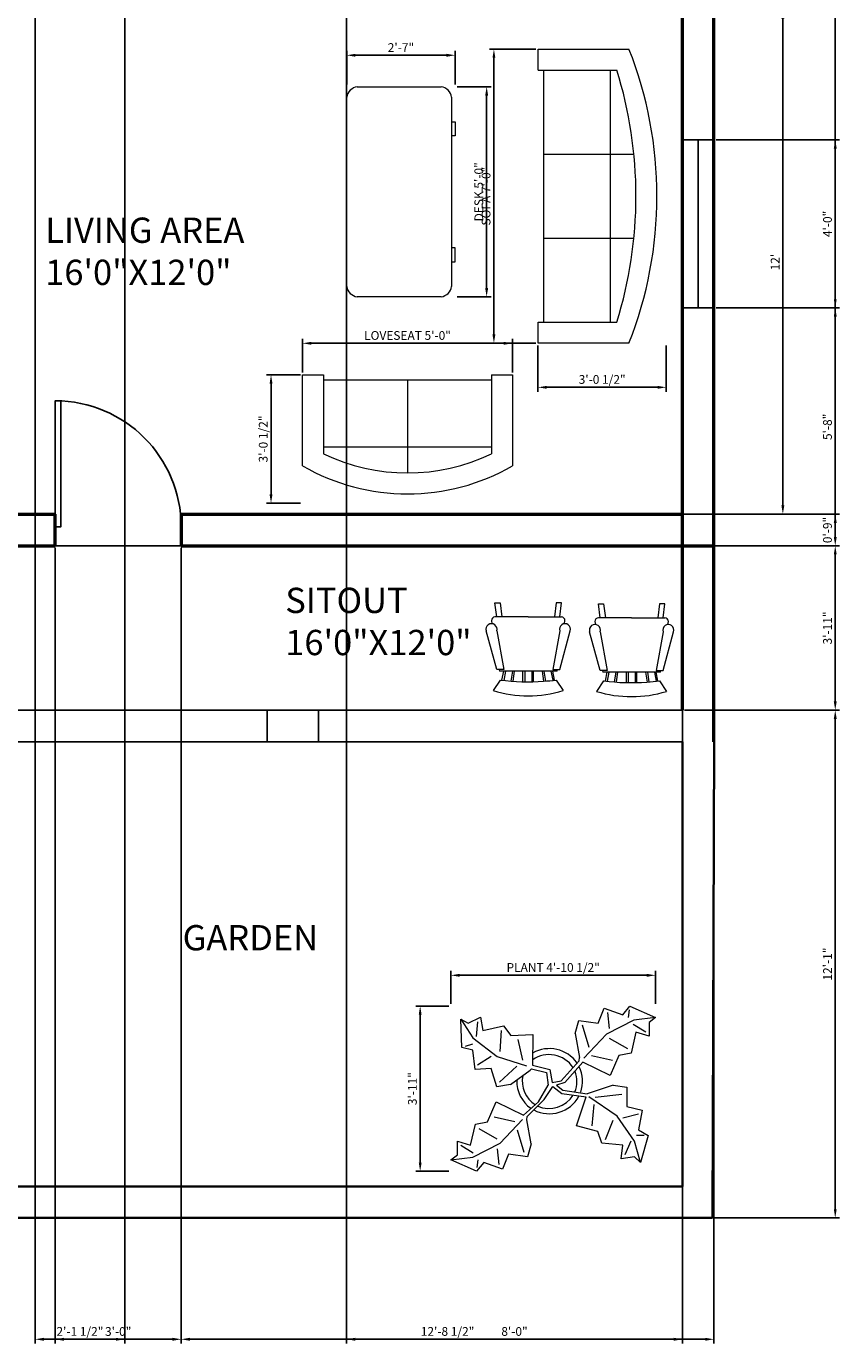
# Model space of a CAD drawing. Units: inches. Extents: x 25547 to 25983, y 30413 to 31159.
# Tile 2 of 5: x 25750 to 25982, y 30413 to 30790. Entities that reach past the tile are written whole.
import ezdxf

# ---------------------------------------------------------------- set-up
doc = ezdxf.new("R2010")
doc.units = ezdxf.units.IN
for name, color, linetype, lineweight in [('A-AREA-IDEN', 11, 'Continuous', 25), ('A-FLOR-PORC', 151, 'Continuous', 25), ('A-WALL', 7, 'Continuous', 50), ('DIM', 4, 'Continuous', 18), ('DOOR', 3, 'Continuous', 25), ('FLOWER', 60, 'Continuous', 13), ('FURNITURES', 6, 'Continuous', 18), ('L-SITE-WALL', 7, 'Continuous', 35), ('WINDOW', 1, 'Continuous', 25)]:
    doc.layers.add(name, color=color, linetype=linetype, lineweight=lineweight)
doc.styles.get("Standard").update_dxf_attribs({"font": 'arial.ttf'})
doc.dimstyles.new('ISO-25', dxfattribs={"dimtxt": 2.5, "dimasz": 2.5, "dimexe": 1.25, "dimexo": 0.625, "dimtad": 1, "dimlunit": 3, "dimtxsty": 'Standard', "dimcen": 2.5, "dimadec": 0, "dimazin": 0, "dimtfac": 1, "dimtmove": 0, "dimatfit": 3, "dimfxl": 1, "dimarcsym": 0})

# ---------------------------------------------------------------- blocks, each defined once
blk = doc.blocks.new('*U2')
for p, q in [((0, 0), (0, -6)), ((40, 0), (40, -6))]:
    blk.add_line(p, q)
blk.add_lwpolyline([(0, 0), (0, 40), (1.75, 40), (1.75, 0)], close=True)
blk.add_arc((0, 0), 40, 0, 90)
blk = doc.blocks.new('Desk - 30 x 60 in.')
for p, q in [((-26.999995, 0), (26.999995, 0)), ((-29.999995, -27), (-29.999995, -3)), ((29.999995, -3), (29.999995, -27)), ((26.999995, -30), (-26.999995, -30)), ((-20.000005, -30), (-20.000005, -31)), ((-16.000005, -31), (-16.000005, -30)), ((15.999995, -31), (15.999995, -30)), ((19.999995, -30), (19.999995, -31)), ((-20.000005, -31), (-16.000005, -31)), ((19.999995, -31), (15.999995, -31))]:
    blk.add_line(p, q)
for centre, start, end in [((-26.499995, -3.5), 98.1301, 171.8699), ((26.499995, -3.5), 8.130102, 81.8699), ((-26.499995, -26.5), 188.1301, 261.8699), ((26.499995, -26.5), 278.1301, 351.8699)]:
    blk.add_arc(centre, 3.535534, start, end)
blk = doc.blocks.new('Sofa - Roundback 7 ft.')
for p, q in [((-12.00002, -32.4421), (-12.00003, -6.5971)), ((11.99997, -32.4421), (11.99998, -6.5971)), ((-36.000027, -34), (-36.000027, -11.4696)), ((-35.999844, -13.3819), (35.9998, -13.3819)), ((35.99998, -34), (35.99998, -11.4696)), ((-36.000027, -32.4421), (35.99998, -32.4421))]:
    blk.add_line(p, q)
for points in [[(-36.000027, -34), (-42.000027, -34), (-42.000027, -8)], [(41.99998, -8), (41.99998, -34), (35.99998, -34)]]:
    blk.add_lwpolyline(points)
for centre, radius, start, end in [((0, -114.25), 114.25, 68.43141, 111.5686), ((-0.00001, -127.1968), 121.1968, 72.72033, 107.2797)]:
    blk.add_arc(centre, radius, start, end)
blk = doc.blocks.new('Sofa - Roundback Loveseat 5 ft.')
for p, q in [((0, -32.44198), (0, -5.99998)), ((-24, -33.99998), (-24, -11.46958)), ((-23.9998, -13.38178), (23.99986, -13.38178)), ((24.00004, -33.99998), (24.00004, -11.46958)), ((-24, -32.44198), (24.00004, -32.44198))]:
    blk.add_line(p, q)
for points in [[(-24, -33.99998), (-30, -33.99998), (-30, -7.99998)], [(30.00004, -7.99998), (30.00004, -33.99998), (24.00004, -33.99998)]]:
    blk.add_lwpolyline(points)
for centre, radius, start, end in [((0, -60.24998), 60.24998, 60.13715, 119.8628), ((0, -61.38438), 55.38444, 64.32083, 115.6792)]:
    blk.add_arc(centre, radius, start, end)
blk = doc.blocks.new('Plant - Rubber or Philodendron')
for p, q in [((8.8871, 10.7908), (9.9809, 13.4933)), ((9.9809, 13.4933), (13.3837, 12.301)), ((10.5828, 12.6946), (10.8893, 9.7953)), ((13.3837, 12.301), (14.68, 13.9039)), ((14.5816, 13.2037), (14.3848, 11.8033)), ((14.68, 13.9039), (19.3848, 11.8146)), ((-16.2005, 11.4774), (-13.9899, 8.1064)), ((-16.2005, 11.4774), (-14.8639, 10.7964)), ((-16.0159, 6.3329), (-16.2005, 11.4774)), ((-14.8639, 10.7964), (-12.6195, 11.8975)), ((-13.3174, 8.325), (-13.0735, 11.0065)), ((-12.6195, 11.8975), (-12.1909, 9.4345)), ((-12.1909, 9.4345), (-8.3829, 10.3)), ((-8.3829, 10.3), (-7.0549, 8.501)), ((4.6914, 8.8812), (5.3859, 11.2828)), ((5.3859, 11.2828), (8.8871, 10.7908)), ((5.9878, 10.4842), (7.1971, 6.3869)), ((15.3859, 11.3055), (10.3916, 8.7942)), ((15.2875, 10.6053), (17.5907, 9.2105)), ((19.3848, 11.8146), (15.3859, 11.3055)), ((19.3848, 11.8146), (18.1868, 10.9119)), ((18.1868, 10.9119), (18.1925, 8.4119)), ((-13.9899, 8.1064), (-9.5434, 4.7185)), ((-8.8369, 9.409), (-9.0894, 5.6095)), ((-7.0549, 8.501), (-3.0284, 8.6941)), ((-4.8529, 4.012), (-5.7184, 7.82)), ((-3.0284, 8.6941), (-3.0709, 3.1041)), ((4.6914, 8.8812), (5.5014, 4.4831)), ((10.3916, 8.7942), (6.2847, 4.4028)), ((14.2977, 6.1031), (10.9934, 7.9956)), ((15.7909, 9.1065), (14.8995, 5.3044)), ((18.1925, 8.4119), (15.7909, 9.1065)), ((-14.0069, 5.8704), (-16.0159, 6.3329)), ((-15.3434, 6.5514), (-13.9984, 6.9884)), ((-13.5868, 2.2894), (-14.0069, 5.8704)), ((7.7005, 4.8881), (11.5025, 3.9967)), ((12.7005, 4.8994), (11.1089, 1.1958)), ((14.8995, 5.3044), (12.7005, 4.8994)), ((-10.6784, 2.491), (-13.5868, 2.2894)), ((-13.1329, 3.1804), (-10.6614, 4.727)), ((-9.5858, -0.8715), (-10.6784, 2.491)), ((-9.5434, 4.7185), (-4.1917, 2.9888)), ((-9.1318, 0.0195), (-5.9793, 2.9025)), ((-3.5248, 2.2131), (-3.3011, 2.4355)), ((-3.3011, 2.4355), (-0.5306, 1.7947)), ((-3.0709, 3.1041), (0.0797, 2.3163)), ((2.1141, 0.2298), (5.4346, 3.9146)), ((6.1032, 3.6844), (2.8262, -0.031)), ((5.4346, 3.9146), (5.5014, 4.4831)), ((11.1089, 1.1958), (6.1032, 3.6844)), ((-7.1228, -0.443), (-3.5248, 2.2131)), ((-0.5306, 1.7947), (-0.2255, -0.5527)), ((-0.5306, 1.7947), (-0.5306, 1.7947)), ((0.0797, 2.3163), (0.4866, -0.031)), ((0.4866, -0.031), (2.1141, 0.2298)), ((-7.1228, -0.443), (-9.5858, -0.8715)), ((-2.019, -3.6148), (-0.2255, -0.5527)), ((-0.9375, -3.1608), (0.5883, -0.8135)), ((0.5883, -0.8135), (2.2447, -2.0916)), ((2.8262, -0.031), (1.3003, -0.5527)), ((1.3003, -0.5527), (2.4193, -1.4655)), ((2.2447, -2.0916), (6.7108, -2.6626)), ((2.4193, -1.4655), (6.895, -2.1175)), ((11.6605, -0.5413), (6.895, -2.1175)), ((8.3544, -2.7453), (13.1973, -2.1704)), ((11.6605, -0.5413), (14.1354, -0.8948)), ((14.1354, -0.8948), (14.1354, -4.4304)), ((-11.3237, -7.2629), (-9.7321, -3.5593)), ((-9.7321, -3.5593), (-4.7264, -6.0479)), ((-2.019, -3.6148), (-4.7264, -6.0479)), ((-4.0579, -6.2781), (-0.9375, -3.1608)), ((4.943, -7.9659), (6.7108, -2.6626)), ((12.3677, -6.1981), (7.219, -2.6772)), ((8.125, -4.0768), (7.7715, -7.9659)), ((14.1354, -4.4304), (16.9638, -5.1375)), ((-6.3237, -7.2516), (-10.1257, -6.3602)), ((-9.0148, -11.1577), (-4.9047, -6.8122)), ((-4.1246, -6.8466), (-4.0579, -6.2781)), ((-3.3146, -11.2447), (-4.1246, -6.8466)), ((10.2463, -10.4408), (11.6605, -6.9053)), ((15.5496, -10.7943), (12.3677, -6.1981)), ((16.2567, -5.8446), (13.4283, -6.5517)), ((16.9638, -5.1375), (16.2567, -8.673)), ((-14.4141, -11.4699), (-13.5228, -7.6679)), ((-13.5228, -7.6679), (-11.3237, -7.2629)), ((-12.921, -8.4665), (-9.6166, -10.359)), ((-4.611, -12.8477), (-5.8203, -8.7504)), ((8.8321, -9.0266), (4.943, -7.9659)), ((9.5392, -11.1479), (8.8321, -9.0266)), ((16.2567, -8.673), (18.0245, -9.7337)), ((-16.8157, -10.7754), (-14.4141, -11.4699)), ((-16.8101, -13.2754), (-16.8157, -10.7754)), ((-13.9107, -12.9688), (-16.2139, -11.574)), ((-14.0091, -13.669), (-9.0148, -11.1577)), ((-3.3146, -11.2447), (-4.0092, -13.6463)), ((13.4283, -11.5015), (9.5392, -11.1479)), ((13.0748, -13.9763), (13.4283, -11.5015)), ((14.8425, -10.7943), (13.7819, -13.2692)), ((16.6103, -14.6834), (15.5496, -10.7943)), ((17.3174, -9.7337), (15.9032, -9.7337)), ((18.0245, -9.7337), (16.6103, -14.6834)), ((-18.008, -14.1781), (-16.8101, -13.2754)), ((-18.008, -14.1781), (-14.0091, -13.669)), ((-13.3032, -16.2674), (-18.008, -14.1781)), ((-13.2048, -15.5672), (-13.008, -14.1668)), ((-9.206, -15.0581), (-9.5126, -12.1588)), ((-7.5103, -13.1543), (-8.6042, -15.8568)), ((-4.0092, -13.6463), (-7.5103, -13.1543)), ((15.5496, -13.6228), (13.0748, -13.9763)), ((16.6103, -14.6834), (15.5496, -13.6228)), ((-12.0069, -14.6645), (-13.3032, -16.2674)), ((-8.6042, -15.8568), (-12.0069, -14.6645))]:
    blk.add_line(p, q)
for centre, radius, start, end in [((0, 0), 6.1275, 34.37569, 120.1028), ((-0.0601, -0.2075), 5.2461, 33.82192, 124.9414), ((-0.098, 0.1364), 6.1288, 341.2017, 26.09184), ((0.0308, 0.1664), 6, 178.6147, 235.1169), ((0.0308, 0.1664), 5, 168.1647, 238.6725), ((-0.2664, 0.1682), 5.2775, 338.4094, 20.03007), ((-0.1102, 0.4886), 5.2883, 247.3711, 327.472), ((-0.0234, 0.3825), 6.1492, 242.5812, 331.2714)]:
    blk.add_arc(centre, radius, start, end)
blk = doc.blocks.new('Chair - Rocking')
for p, q in [((-8, -4.5), (-10, -1.5)), ((8, -4.5), (10, -1.5)), ((-9, -7.5), (-12, -18.49999)), ((-7, -7.5), (-9, -7.5)), ((-9, -18.49999), (-7, -7.5)), ((-8.23428, -6.99939), (-8.3093, -7.47958)), ((-8.23041, -7), (8.23915, -7)), ((-7.5, -4.5), (-7, -7)), ((-6.5, -7), (-7.02225, -4.43)), ((-4.5, -7), (-4.96674, -4.19951)), ((-4, -7), (-4.40532, -4.16272)), ((-1.5, -4.05012), (-1.5, -7)), ((-1, -7), (-1, -4.05012)), ((1, -7), (1, -4.04655)), ((1.5, -4.05012), (1.5, -7)), ((4, -7), (4.40187, -4.18694)), ((4.5, -7), (4.96761, -4.19437)), ((6.5, -7), (7, -4.4057)), ((7.5, -4.5), (7, -7)), ((7, -7.5), (9, -7.5)), ((9, -18.49999), (7, -7.5)), ((8.31071, -7.48854), (8.23449, -7.00073)), ((9, -7.5), (12, -18.49999)), ((-10.36644, -20.64523), (-10.5, -21.49999)), ((-9, -22.49999), (-9.5, -26.49999)), ((0, -22.49999), (-9.5, -22.49999)), ((-8, -26.49999), (-7.5, -22.49999)), ((0, -22.49999), (9.5, -22.49999)), ((8, -26.49999), (7.5, -22.49999)), ((9, -22.49999), (9.5, -26.49999)), ((10.5, -21.49999), (10.3575, -20.58798)), ((-9.5, -26.49999), (-8, -26.49999)), ((9.5, -26.49999), (8, -26.49999))]:
    blk.add_line(p, q)
for centre, radius, start, end in [((0, -34.08333), 34.08333, 72.93847, 107.0615), ((0, -68.25004), 64.25, 93.92211, 97.15267), ((0, -68.25004), 64.25, 82.84733, 93.92211), ((-10.5, -18.99999), 1.58114, 161.5651, 18.43495), ((10.5, -18.99999), 1.58114, 161.5651, 18.43495), ((-9.5, -21.49999), 1, 180, 270), ((9.5, -21.49999), 1, 270, 0)]:
    blk.add_arc(centre, radius, start, end)
blk = doc.blocks.new('*D28')
at = {"layer": 'Defpoints', "color": 0, "transparency": 16777216}
for p in [(25937.53, 30794.83), (25966.22, 30794.83), (25937.53, 30650.83)]:
    blk.add_point(p, dxfattribs=at)
at = {"layer": 'DIM', "color": 0, "lineweight": -2, "transparency": 16777216}
for p, q in [((25938.15, 30794.83), (25967.47, 30794.83)), ((25966.22, 30653.33), (25966.22, 30792.33)), ((25938.15, 30650.83), (25967.47, 30650.83))]:
    blk.add_line(p, q, dxfattribs=at)
at = {"layer": 'DIM', "color": 0, "transparency": 16777216}
for points in [[(25965.8, 30792.33), (25966.63, 30792.33), (25966.22, 30794.83)], [(25965.8, 30653.33), (25966.63, 30653.33), (25966.22, 30650.83)]]:
    blk.add_solid(points, dxfattribs=at)
at = {"layer": 'DIM', "color": 0, "transparency": 16777216, "insert": (25964.34, 30722.83), "char_height": 2.5, "attachment_point": 5, "rotation": 90}
blk.add_mtext("12'", dxfattribs=at)
blk = doc.blocks.new('WIN-48IN')
blk.add_line((4.5, 48), (4.5, 0))
blk.add_lwpolyline([(0, 48), (9, 48), (9, 0), (0, 0)], close=True)
blk = doc.blocks.new('*D48')
at = {"layer": 'Defpoints', "color": 0, "transparency": 16777216}
for p in [(25929.84, 30519.14), (25871.35, 30510.37), (25929.84, 30510.37)]:
    blk.add_point(p, dxfattribs=at)
at = {"layer": 'DIM', "color": 0, "lineweight": -2, "transparency": 16777216}
for p, q in [((25871.35, 30510.99), (25871.35, 30520.39)), ((25929.84, 30510.99), (25929.84, 30520.39)), ((25873.85, 30519.14), (25927.34, 30519.14))]:
    blk.add_line(p, q, dxfattribs=at)
at = {"layer": 'DIM', "color": 0, "transparency": 16777216}
for points in [[(25873.85, 30519.56), (25873.85, 30518.72), (25871.35, 30519.14)], [(25927.34, 30519.56), (25927.34, 30518.72), (25929.84, 30519.14)]]:
    blk.add_solid(points, dxfattribs=at)
at = {"layer": 'DIM', "color": 0, "transparency": 16777216, "insert": (25900.59, 30521.06), "char_height": 2.5, "attachment_point": 5}
blk.add_mtext('PLANT 4\'-10 1/2"', dxfattribs=at)
blk = doc.blocks.new('*D49')
at = {"layer": 'Defpoints', "color": 0, "transparency": 16777216}
for p in [(25862.57, 30510.37), (25871.35, 30510.37), (25871.35, 30463.17)]:
    blk.add_point(p, dxfattribs=at)
at = {"layer": 'DIM', "color": 0, "lineweight": -2, "transparency": 16777216}
for p, q in [((25870.72, 30510.37), (25861.32, 30510.37)), ((25862.57, 30465.67), (25862.57, 30507.87)), ((25870.72, 30463.17), (25861.32, 30463.17))]:
    blk.add_line(p, q, dxfattribs=at)
at = {"layer": 'DIM', "color": 0, "transparency": 16777216}
for points in [[(25862.16, 30507.87), (25862.99, 30507.87), (25862.57, 30510.37)], [(25862.16, 30465.67), (25862.99, 30465.67), (25862.57, 30463.17)]]:
    blk.add_solid(points, dxfattribs=at)
at = {"layer": 'DIM', "color": 0, "transparency": 16777216, "insert": (25860.67, 30486.77), "char_height": 2.5, "attachment_point": 5, "rotation": 90}
blk.add_mtext('3\'-11"', dxfattribs=at)
blk = doc.blocks.new('*D58')
at = {"layer": 'Defpoints', "color": 0, "transparency": 16777216}
for p in [(25872.57, 30772.91), (25881.57, 30772.91), (25872.57, 30712.91)]:
    blk.add_point(p, dxfattribs=at)
at = {"layer": 'DIM', "color": 0, "lineweight": -2, "transparency": 16777216}
for p, q in [((25873.19, 30772.91), (25882.82, 30772.91)), ((25881.57, 30715.41), (25881.57, 30770.41)), ((25873.19, 30712.91), (25882.82, 30712.91))]:
    blk.add_line(p, q, dxfattribs=at)
at = {"layer": 'DIM', "color": 0, "transparency": 16777216}
for points in [[(25881.15, 30770.41), (25881.99, 30770.41), (25881.57, 30772.91)], [(25881.15, 30715.41), (25881.99, 30715.41), (25881.57, 30712.91)]]:
    blk.add_solid(points, dxfattribs=at)
at = {"layer": 'DIM', "color": 0, "transparency": 16777216, "insert": (25879.65, 30742.91), "char_height": 2.5, "attachment_point": 5, "rotation": 90}
blk.add_mtext('DESK 5\'-0"', dxfattribs=at)
blk = doc.blocks.new('*D59')
at = {"layer": 'Defpoints', "color": 0, "transparency": 16777216}
for p in [(25841.57, 30781.91), (25841.57, 30772.91), (25872.57, 30772.91)]:
    blk.add_point(p, dxfattribs=at)
at = {"layer": 'DIM', "color": 0, "lineweight": -2, "transparency": 16777216}
for p, q in [((25841.57, 30773.53), (25841.57, 30783.16)), ((25872.57, 30773.53), (25872.57, 30783.16)), ((25870.07, 30781.91), (25844.07, 30781.91))]:
    blk.add_line(p, q, dxfattribs=at)
at = {"layer": 'DIM', "color": 0, "transparency": 16777216}
for points in [[(25844.07, 30782.33), (25844.07, 30781.49), (25841.57, 30781.91)], [(25870.07, 30782.33), (25870.07, 30781.49), (25872.57, 30781.91)]]:
    blk.add_solid(points, dxfattribs=at)
at = {"layer": 'DIM', "color": 0, "transparency": 16777216, "insert": (25857.07, 30783.79), "char_height": 2.5, "attachment_point": 5}
blk.add_mtext('2\'-7"', dxfattribs=at)
blk = doc.blocks.new('*D62')
at = {"layer": 'Defpoints', "color": 0, "transparency": 16777216}
for p in [(25896.24, 30783.68), (25883.64, 30699.68), (25896.24, 30699.68)]:
    blk.add_point(p, dxfattribs=at)
at = {"layer": 'DIM', "color": 0, "lineweight": -2, "transparency": 16777216}
for p, q in [((25895.62, 30783.68), (25882.39, 30783.68)), ((25883.64, 30781.18), (25883.64, 30702.18)), ((25895.62, 30699.68), (25882.39, 30699.68))]:
    blk.add_line(p, q, dxfattribs=at)
at = {"layer": 'DIM', "color": 0, "transparency": 16777216}
for points in [[(25883.23, 30781.18), (25884.06, 30781.18), (25883.64, 30783.68)], [(25883.23, 30702.18), (25884.06, 30702.18), (25883.64, 30699.68)]]:
    blk.add_solid(points, dxfattribs=at)
at = {"layer": 'DIM', "color": 0, "transparency": 16777216, "insert": (25881.73, 30741.68), "char_height": 2.5, "attachment_point": 5, "rotation": 90}
blk.add_mtext('SOFA 7\'-0"', dxfattribs=at)
blk = doc.blocks.new('*D63')
at = {"layer": 'Defpoints', "color": 0, "transparency": 16777216}
for p in [(25896.24, 30699.68), (25932.91, 30699.68), (25932.91, 30687.08)]:
    blk.add_point(p, dxfattribs=at)
at = {"layer": 'DIM', "color": 0, "lineweight": -2, "transparency": 16777216}
for p, q in [((25896.24, 30699.05), (25896.24, 30685.83)), ((25932.91, 30699.05), (25932.91, 30685.83)), ((25898.74, 30687.08), (25930.41, 30687.08))]:
    blk.add_line(p, q, dxfattribs=at)
at = {"layer": 'DIM', "color": 0, "transparency": 16777216}
for points in [[(25898.74, 30687.49), (25898.74, 30686.66), (25896.24, 30687.08)], [(25930.41, 30687.49), (25930.41, 30686.66), (25932.91, 30687.08)]]:
    blk.add_solid(points, dxfattribs=at)
at = {"layer": 'DIM', "color": 0, "transparency": 16777216, "insert": (25914.58, 30689), "char_height": 2.5, "attachment_point": 5}
blk.add_mtext('3\'-0 1/2"', dxfattribs=at)
blk = doc.blocks.new('*D64')
at = {"layer": 'Defpoints', "color": 0, "transparency": 16777216}
for p in [(25828.95, 30699.64), (25828.95, 30690.64), (25888.95, 30690.64)]:
    blk.add_point(p, dxfattribs=at)
at = {"layer": 'DIM', "color": 0, "lineweight": -2, "transparency": 16777216}
for p, q in [((25828.95, 30691.27), (25828.95, 30700.89)), ((25888.95, 30691.27), (25888.95, 30700.89)), ((25886.45, 30699.64), (25831.45, 30699.64))]:
    blk.add_line(p, q, dxfattribs=at)
at = {"layer": 'DIM', "color": 0, "transparency": 16777216}
for points in [[(25831.45, 30700.06), (25831.45, 30699.23), (25828.95, 30699.64)], [(25886.45, 30700.06), (25886.45, 30699.23), (25888.95, 30699.64)]]:
    blk.add_solid(points, dxfattribs=at)
at = {"layer": 'DIM', "color": 0, "transparency": 16777216, "insert": (25858.95, 30701.56), "char_height": 2.5, "attachment_point": 5}
blk.add_mtext('LOVESEAT 5\'-0"', dxfattribs=at)
blk = doc.blocks.new('*D65')
at = {"layer": 'Defpoints', "color": 0, "transparency": 16777216}
for p in [(25828.95, 30690.64), (25819.95, 30653.98), (25828.95, 30653.98)]:
    blk.add_point(p, dxfattribs=at)
at = {"layer": 'DIM', "color": 0, "lineweight": -2, "transparency": 16777216}
for p, q in [((25828.33, 30690.64), (25818.7, 30690.64)), ((25819.95, 30688.14), (25819.95, 30656.48)), ((25828.33, 30653.98), (25818.7, 30653.98))]:
    blk.add_line(p, q, dxfattribs=at)
at = {"layer": 'DIM', "color": 0, "transparency": 16777216}
for points in [[(25819.54, 30688.14), (25820.37, 30688.14), (25819.95, 30690.64)], [(25819.54, 30656.48), (25820.37, 30656.48), (25819.95, 30653.98)]]:
    blk.add_solid(points, dxfattribs=at)
at = {"layer": 'DIM', "color": 0, "transparency": 16777216, "insert": (25818.04, 30672.31), "char_height": 2.5, "attachment_point": 5, "rotation": 90}
blk.add_mtext('3\'-0 1/2"', dxfattribs=at)
blk = doc.blocks.new('*D69')
at = {"layer": 'Defpoints', "color": 0, "transparency": 16777216}
for p in [(25937.53, 30594.87), (25981.19, 30594.87), (25946.13, 30449.83)]:
    blk.add_point(p, dxfattribs=at)
at = {"layer": 'DIM', "color": 0, "lineweight": -2, "transparency": 16777216}
for p, q in [((25938.15, 30594.87), (25982.44, 30594.87)), ((25981.19, 30452.33), (25981.19, 30592.37)), ((25946.76, 30449.83), (25982.44, 30449.83))]:
    blk.add_line(p, q, dxfattribs=at)
at = {"layer": 'DIM', "color": 0, "transparency": 16777216}
for points in [[(25980.78, 30592.37), (25981.61, 30592.37), (25981.19, 30594.87)], [(25980.78, 30452.33), (25981.61, 30452.33), (25981.19, 30449.83)]]:
    blk.add_solid(points, dxfattribs=at)
at = {"layer": 'DIM', "color": 0, "transparency": 16777216, "insert": (25979.31, 30522.35), "char_height": 2.5, "attachment_point": 5, "rotation": 90}
blk.add_mtext('12\'-1"', dxfattribs=at)
blk = doc.blocks.new('*D70')
at = {"layer": 'Defpoints', "color": 0, "transparency": 16777216}
for p in [(25946.53, 31118.83), (25981.19, 31118.83), (25946.53, 30641.83)]:
    blk.add_point(p, dxfattribs=at)
at = {"layer": 'DIM', "color": 0, "lineweight": -2, "transparency": 16777216}
for p, q in [((25947.15, 31118.83), (25982.44, 31118.83)), ((25981.19, 30644.33), (25981.19, 31116.33)), ((25947.15, 30641.83), (25982.44, 30641.83))]:
    blk.add_line(p, q, dxfattribs=at)
at = {"layer": 'DIM', "color": 0, "transparency": 16777216}
for points in [[(25980.78, 31116.33), (25981.61, 31116.33), (25981.19, 31118.83)], [(25980.78, 30644.33), (25981.61, 30644.33), (25981.19, 30641.83)]]:
    blk.add_solid(points, dxfattribs=at)
at = {"layer": 'DIM', "color": 0, "transparency": 16777216, "insert": (25979.29, 30880.33), "char_height": 2.5, "attachment_point": 5, "rotation": 90}
blk.add_mtext('39\'-9"', dxfattribs=at)
blk = doc.blocks.new('*D83')
at = {"layer": 'Defpoints', "color": 0, "transparency": 16777216}
for p in [(25841.53, 30847.83), (25937.53, 30799.83), (25937.53, 30415.19)]:
    blk.add_point(p, dxfattribs=at)
at = {"layer": 'DIM', "color": 0, "lineweight": -2, "transparency": 16777216}
for p, q in [((25841.53, 30847.2), (25841.53, 30413.94)), ((25937.53, 30799.2), (25937.53, 30413.94)), ((25844.03, 30415.19), (25935.03, 30415.19))]:
    blk.add_line(p, q, dxfattribs=at)
at = {"layer": 'DIM', "color": 0, "transparency": 16777216}
for points in [[(25844.03, 30415.61), (25844.03, 30414.77), (25841.53, 30415.19)], [(25935.03, 30415.61), (25935.03, 30414.77), (25937.53, 30415.19)]]:
    blk.add_solid(points, dxfattribs=at)
at = {"layer": 'DIM', "color": 0, "transparency": 16777216, "insert": (25889.53, 30417.09), "char_height": 2.5, "attachment_point": 5}
blk.add_mtext('8\'-0"', dxfattribs=at)
blk = doc.blocks.new('*D86')
at = {"layer": 'Defpoints', "color": 0, "transparency": 16777216}
for p in [(25946.53, 30709.75), (25946.53, 30641.83), (25981.19, 30641.83)]:
    blk.add_point(p, dxfattribs=at)
at = {"layer": 'DIM', "color": 0, "lineweight": -2, "transparency": 16777216}
for p, q in [((25947.15, 30709.75), (25982.44, 30709.75)), ((25981.19, 30707.25), (25981.19, 30644.33)), ((25947.15, 30641.83), (25982.44, 30641.83))]:
    blk.add_line(p, q, dxfattribs=at)
at = {"layer": 'DIM', "color": 0, "transparency": 16777216}
for points in [[(25980.78, 30707.25), (25981.61, 30707.25), (25981.19, 30709.75)], [(25980.78, 30644.33), (25981.61, 30644.33), (25981.19, 30641.83)]]:
    blk.add_solid(points, dxfattribs=at)
at = {"layer": 'DIM', "color": 0, "transparency": 16777216, "insert": (25979.29, 30675.79), "char_height": 2.5, "attachment_point": 5, "rotation": 90}
blk.add_mtext('5\'-8"', dxfattribs=at)
blk = doc.blocks.new('*D87')
at = {"layer": 'Defpoints', "color": 0, "transparency": 16777216}
for p in [(25946.53, 30641.83), (25981.19, 30641.83), (25937.53, 30594.87)]:
    blk.add_point(p, dxfattribs=at)
at = {"layer": 'DIM', "color": 0, "lineweight": -2, "transparency": 16777216}
for p, q in [((25947.15, 30641.83), (25982.44, 30641.83)), ((25981.19, 30597.37), (25981.19, 30639.33)), ((25938.15, 30594.87), (25982.44, 30594.87))]:
    blk.add_line(p, q, dxfattribs=at)
at = {"layer": 'DIM', "color": 0, "transparency": 16777216}
for points in [[(25980.78, 30639.33), (25981.61, 30639.33), (25981.19, 30641.83)], [(25980.78, 30597.37), (25981.61, 30597.37), (25981.19, 30594.87)]]:
    blk.add_solid(points, dxfattribs=at)
at = {"layer": 'DIM', "color": 0, "transparency": 16777216, "insert": (25979.29, 30618.35), "char_height": 2.5, "attachment_point": 5, "rotation": 90}
blk.add_mtext('3\'-11"', dxfattribs=at)
blk = doc.blocks.new('*D88')
at = {"layer": 'Defpoints', "color": 0, "transparency": 16777216}
for p in [(25758.27, 30641.83), (25794.27, 30641.83), (25794.27, 30415.19)]:
    blk.add_point(p, dxfattribs=at)
at = {"layer": 'DIM', "color": 0, "lineweight": -2, "transparency": 16777216}
for p, q in [((25758.27, 30641.2), (25758.27, 30413.94)), ((25794.27, 30641.2), (25794.27, 30413.94)), ((25760.77, 30415.19), (25791.77, 30415.19))]:
    blk.add_line(p, q, dxfattribs=at)
at = {"layer": 'DIM', "color": 0, "transparency": 16777216}
for points in [[(25760.77, 30415.61), (25760.77, 30414.77), (25758.27, 30415.19)], [(25791.77, 30415.61), (25791.77, 30414.77), (25794.27, 30415.19)]]:
    blk.add_solid(points, dxfattribs=at)
at = {"layer": 'DIM', "color": 0, "transparency": 16777216, "insert": (25776.27, 30417.09), "char_height": 2.5, "attachment_point": 5}
blk.add_mtext('3\'-0"', dxfattribs=at)
blk = doc.blocks.new('*D89')
at = {"layer": 'Defpoints', "color": 0, "transparency": 16777216}
for p in [(25794.27, 30641.83), (25946.53, 30641.83), (25946.53, 30415.19)]:
    blk.add_point(p, dxfattribs=at)
at = {"layer": 'DIM', "color": 0, "lineweight": -2, "transparency": 16777216}
for p, q in [((25794.27, 30641.2), (25794.27, 30413.94)), ((25946.53, 30641.2), (25946.53, 30413.94)), ((25796.77, 30415.19), (25944.03, 30415.19))]:
    blk.add_line(p, q, dxfattribs=at)
at = {"layer": 'DIM', "color": 0, "transparency": 16777216}
for points in [[(25796.77, 30415.61), (25796.77, 30414.77), (25794.27, 30415.19)], [(25944.03, 30415.61), (25944.03, 30414.77), (25946.53, 30415.19)]]:
    blk.add_solid(points, dxfattribs=at)
at = {"layer": 'DIM', "color": 0, "transparency": 16777216, "insert": (25870.4, 30417.11), "char_height": 2.5, "attachment_point": 5}
blk.add_mtext('12\'-8 1/2"', dxfattribs=at)
blk = doc.blocks.new('*D94')
at = {"layer": 'Defpoints', "color": 0, "transparency": 16777216}
for p in [(25946.53, 30757.75), (25981.19, 30757.75), (25946.53, 30709.75)]:
    blk.add_point(p, dxfattribs=at)
at = {"layer": 'DIM', "color": 0, "lineweight": -2, "transparency": 16777216}
for p, q in [((25947.15, 30757.75), (25982.44, 30757.75)), ((25981.19, 30712.25), (25981.19, 30755.25)), ((25947.15, 30709.75), (25982.44, 30709.75))]:
    blk.add_line(p, q, dxfattribs=at)
at = {"layer": 'DIM', "color": 0, "transparency": 16777216}
for points in [[(25980.78, 30755.25), (25981.61, 30755.25), (25981.19, 30757.75)], [(25980.78, 30712.25), (25981.61, 30712.25), (25981.19, 30709.75)]]:
    blk.add_solid(points, dxfattribs=at)
at = {"layer": 'DIM', "color": 0, "transparency": 16777216, "insert": (25979.29, 30733.75), "char_height": 2.5, "attachment_point": 5, "rotation": 90}
blk.add_mtext('4\'-0"', dxfattribs=at)
blk = doc.blocks.new('*D102')
at = {"layer": 'Defpoints', "color": 0, "transparency": 16777216}
for p in [(25794.27, 30650.83), (25981.19, 30650.83), (25794.27, 30641.83)]:
    blk.add_point(p, dxfattribs=at)
at = {"layer": 'DIM', "color": 0, "lineweight": -2, "transparency": 16777216}
for p, q in [((25794.9, 30650.83), (25982.44, 30650.83)), ((25981.19, 30644.33), (25981.19, 30648.33)), ((25794.9, 30641.83), (25982.44, 30641.83))]:
    blk.add_line(p, q, dxfattribs=at)
at = {"layer": 'DIM', "color": 0, "transparency": 16777216}
for points in [[(25980.78, 30648.33), (25981.61, 30648.33), (25981.19, 30650.83)], [(25980.78, 30644.33), (25981.61, 30644.33), (25981.19, 30641.83)]]:
    blk.add_solid(points, dxfattribs=at)
at = {"layer": 'DIM', "color": 0, "transparency": 16777216, "insert": (25979.29, 30646.33), "char_height": 2.5, "attachment_point": 5, "rotation": 90}
blk.add_mtext('0\'-9"', dxfattribs=at)
blk = doc.blocks.new('*D103')
at = {"layer": 'Defpoints', "color": 0, "transparency": 16777216}
for p in [(25752.53, 31019.83), (25778.13, 31019.83), (25778.13, 30415.19)]:
    blk.add_point(p, dxfattribs=at)
at = {"layer": 'DIM', "color": 0, "lineweight": -2, "transparency": 16777216}
for p, q in [((25752.53, 31019.2), (25752.53, 30413.94)), ((25778.13, 31019.2), (25778.13, 30413.94)), ((25755.03, 30415.19), (25775.63, 30415.19))]:
    blk.add_line(p, q, dxfattribs=at)
at = {"layer": 'DIM', "color": 0, "transparency": 16777216}
for points in [[(25755.03, 30415.61), (25755.03, 30414.77), (25752.53, 30415.19)], [(25775.63, 30415.61), (25775.63, 30414.77), (25778.13, 30415.19)]]:
    blk.add_solid(points, dxfattribs=at)
at = {"layer": 'DIM', "color": 0, "transparency": 16777216, "insert": (25765.33, 30417.11), "char_height": 2.5, "attachment_point": 5}
blk.add_mtext('2\'-1 1/2"', dxfattribs=at)

msp = doc.modelspace()

# ---------------------------------------------------------------- linework, layer by layer
at = {"layer": 'A-FLOR-PORC'}
for p, q in [((25736.247, 30641.828), (25946.557, 30641.828)), ((25937.528, 30594.868), (25716.528, 30594.868)), ((25946.557, 30594.868), (25946.528, 30594.868)), ((25937.528, 30585.868), (25725.528, 30585.868)), ((25946.557, 30585.868), (25946.528, 30585.868))]:
    msp.add_line(p, q, dxfattribs=at)
msp.add_lwpolyline([(25833.473, 30585.868), (25818.841, 30585.868), (25818.841, 30594.868), (25833.473, 30594.868)], close=True, dxfattribs=at)
msp.add_lwpolyline([(25946.528, 30594.868), (25946.557, 30594.868), (25946.557, 30585.868), (25946.528, 30585.868)], dxfattribs=at)
at = {"layer": 'A-WALL'}
for p, q in [((25946.528, 30585.868), (25946.528, 31118.828)), ((25937.528, 30594.868), (25937.528, 31109.828)), ((25596.528, 30650.828), (25758.27, 30650.828)), ((25794.27, 30650.828), (25937.528, 30650.828)), ((25716.528, 30641.828), (25758.27, 30641.828)), ((25794.27, 30641.828), (25946.528, 30641.828))]:
    msp.add_line(p, q, dxfattribs=at)
for points in [[(25758.27, 30641.828), (25758.27, 30650.828)], [(25794.27, 30650.828), (25794.27, 30641.828)]]:
    msp.add_lwpolyline(points, dxfattribs=at)
at = {"layer": 'L-SITE-WALL'}
for p, q in [((25937.528, 30585.868), (25937.528, 30458.828)), ((25946.557, 30585.868), (25946.134, 30449.828)), ((25725.528, 30458.828), (25937.528, 30458.828)), ((25725.528, 30449.828), (25946.134, 30449.828))]:
    msp.add_line(p, q, dxfattribs=at)

# ---------------------------------------------------------------- block references
at = {"layer": 'DOOR', "xscale": 0.9, "yscale": 0.9, "zscale": 0.9}
msp.add_blockref('*U2', (25758.27, 30647.228), dxfattribs=at)
at = {"layer": 'FLOWER', "xscale": 1.564251600455464, "yscale": 1.564251600455464, "zscale": 1.564251600455464}
msp.add_blockref('Plant - Rubber or Philodendron', (25899.517, 30488.617), dxfattribs=at)
at = {"layer": 'FURNITURES'}
for name, p, rotation in [('Sofa - Roundback 7 ft.', (25930.244, 30741.678), 270), ('Desk - 30 x 60 in.', (25841.569, 30742.91), 90), ('Sofa - Roundback Loveseat 5 ft.', (25858.955, 30656.643), 180), ('Chair - Rocking', (25893.454, 30598.981), 180), ('Chair - Rocking', (25922.996, 30598.727), 180)]:
    msp.add_blockref(name, p, dxfattribs=dict(at, rotation=rotation))
at = {"layer": 'WINDOW'}
msp.add_blockref('WIN-48IN', (25937.528, 30709.754), dxfattribs=at)

# ---------------------------------------------------------------- texts
at = {"layer": 'A-AREA-IDEN', "char_height": 7.21917, "attachment_point": 1}
for s, insert in [('{\\fArial|b1|i1|c0|p34;LIVING AREA\\P16\'0"X12\'0"}', (25755.407, 30735.555)), ('{\\fArial|b1|i1|c0|p34;SITOUT\\P16\'0"X12\'0"}', (25824.016, 30629.832)), ('{\\fArial|b1|i1|c0|p34;GARDEN}', (25794.69, 30533.489))]:
    msp.add_mtext_dynamic_manual_height_columns(s, width=113.82935, gutter_width=18.048, heights=[0], dxfattribs=dict(at, insert=insert))

# ---------------------------------------------------------------- dimensions: what is measured, and where the dimension line sits
at = {"layer": 'DIM'}
for base, p1, p2, angle, override, picture, middle in [((25981.195, 31118.828), (25946.528, 30641.828), (25946.528, 31118.828), 90, {"dimdec": 1, "dimlfac": 1, "dimrnd": 0, "dimzin": 1, "dimdsep": 46, "dimlunit": 4, "dimfrac": 2}, '*D70', (25979.292, 30880.328)), ((25966.218, 30794.828), (25937.528, 30650.828), (25937.528, 30794.828), 90, {"dimclrd": 0, "dimclre": 0, "dimclrt": 0}, '*D28', (25964.338, 30722.828)), ((25841.569, 30781.91), (25872.569, 30772.91), (25841.569, 30772.91), 180, {"dimdec": 1, "dimlfac": 1, "dimrnd": 0, "dimzin": 1, "dimdsep": 46, "dimlunit": 4, "dimfrac": 2}, '*D59', (25857.069, 30783.79)), ((25981.195, 30757.754), (25946.528, 30709.754), (25946.528, 30757.754), 90, {"dimdec": 1, "dimlfac": 1, "dimrnd": 0, "dimzin": 1, "dimdsep": 46, "dimlunit": 4, "dimfrac": 2}, '*D94', (25979.293, 30733.754)), ((25981.195, 30641.828), (25946.528, 30709.754), (25946.528, 30641.828), 90, {"dimdec": 1, "dimlfac": 1, "dimrnd": 0, "dimzin": 1, "dimdsep": 46, "dimlunit": 4, "dimfrac": 2}, '*D86', (25979.293, 30675.791)), ((25819.955, 30653.977), (25828.955, 30690.643), (25828.955, 30653.977), 270, {"dimdec": 1, "dimlfac": 1, "dimrnd": 0, "dimzin": 1, "dimdsep": 46, "dimlunit": 4, "dimfrac": 2}, '*D65', (25818.036, 30672.31)), ((25981.195, 30650.828), (25794.27, 30641.828), (25794.27, 30650.828), 90, {"dimdec": 1, "dimlfac": 1, "dimrnd": 0, "dimzin": 1, "dimdsep": 46, "dimlunit": 4, "dimfrac": 2}, '*D102', (25979.293, 30646.328)), ((25981.195, 30641.828), (25937.528, 30594.868), (25946.528, 30641.828), 90, {"dimdec": 1, "dimlfac": 1, "dimrnd": 0, "dimzin": 1, "dimdsep": 46, "dimlunit": 4, "dimfrac": 2}, '*D87', (25979.292, 30618.348)), ((25981.195, 30594.868), (25946.134, 30449.828), (25937.528, 30594.868), 90, {"dimdec": 1, "dimlfac": 1, "dimrnd": 0, "dimzin": 1, "dimdsep": 46, "dimlunit": 4, "dimfrac": 2}, '*D69', (25979.314, 30522.348)), ((25862.574, 30510.366), (25871.348, 30463.171), (25871.348, 30510.366), 90, {"dimdec": 1, "dimlfac": 1, "dimrnd": 0, "dimzin": 1, "dimdsep": 46, "dimlunit": 4, "dimfrac": 2}, '*D49', (25860.672, 30486.769))]:
    dim = msp.add_linear_dim(base=base, p1=p1, p2=p2, angle=angle, dimstyle='ISO-25', override=override, dxfattribs=at)
    dim.commit()
    dim.dimension.update_dxf_attribs({"geometry": picture, "text_midpoint": middle})
for base, p1, p2, picture, middle in [((25778.126, 30415.19), (25752.528, 31019.828), (25778.126, 31019.828), '*D103', (25765.327, 30417.108)), ((25937.528, 30415.19), (25841.528, 30847.828), (25937.528, 30799.828), '*D83', (25889.528, 30417.092)), ((25932.91, 30687.078), (25896.244, 30699.678), (25932.91, 30699.678), '*D63', (25914.577, 30688.996)), ((25794.27, 30415.19), (25758.27, 30641.828), (25794.27, 30641.828), '*D88', (25776.27, 30417.093)), ((25946.528, 30415.19), (25794.27, 30641.828), (25946.528, 30641.828), '*D89', (25870.399, 30417.108))]:
    dim = msp.add_linear_dim(base=base, p1=p1, p2=p2, dimstyle='ISO-25', override={"dimdec": 1, "dimlfac": 1, "dimrnd": 0, "dimzin": 1, "dimdsep": 46, "dimlunit": 4, "dimfrac": 2}, dxfattribs=at)
    dim.commit()
    dim.dimension.update_dxf_attribs({"geometry": picture, "text_midpoint": middle})
for base, p1, p2, angle, text, picture, middle in [((25883.644, 30699.678), (25896.244, 30783.678), (25896.244, 30699.678), 270, 'SOFA <>', '*D62', (25881.725, 30741.678)), ((25881.569, 30772.91), (25872.569, 30712.91), (25872.569, 30772.91), 90, 'DESK <>', '*D58', (25879.651, 30742.91)), ((25828.955, 30699.643), (25888.955, 30690.643), (25828.955, 30690.643), 180, 'LOVESEAT <>', '*D64', (25858.955, 30701.562))]:
    dim = msp.add_linear_dim(base=base, p1=p1, p2=p2, angle=angle, text=text, dimstyle='ISO-25', override={"dimdec": 1, "dimlfac": 1, "dimrnd": 0, "dimzin": 1, "dimdsep": 46, "dimlunit": 4, "dimfrac": 2}, dxfattribs=at)
    dim.commit()
    dim.dimension.update_dxf_attribs({"geometry": picture, "text_midpoint": middle})
dim = msp.add_linear_dim(base=(25929.84, 30519.14), p1=(25871.348, 30510.366), p2=(25929.84, 30510.366), text='PLANT <>', dimstyle='ISO-25', override={"dimdec": 1, "dimlfac": 1, "dimrnd": 0, "dimzin": 1, "dimdsep": 46, "dimlunit": 4, "dimfrac": 2}, dxfattribs=at)
dim.commit()
dim.dimension.update_dxf_attribs({"geometry": '*D48', "text_midpoint": (25900.594, 30521.058)})

doc.saveas('drawing.dxf')
